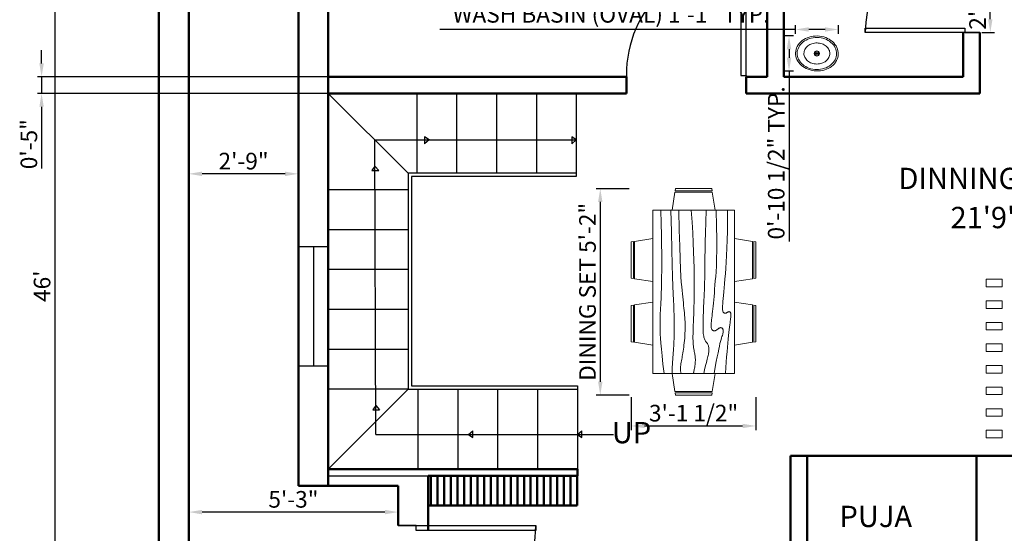
# Model space of a CAD drawing. Units: inches. Extents: x 116541 to 117938, y 135634 to 136328.
# Tile 2 of 9: x 116541 to 116838, y 135936 to 136091. Entities that reach past the tile are written whole.
import ezdxf

# ---------------------------------------------------------------- set-up
doc = ezdxf.new("R2010")
doc.units = ezdxf.units.IN
for name, color, linetype, lineweight in [('A-ANNO-DIMS', 2, 'Continuous', 18), ('A-ANNO-TEXT', 7, 'Continuous', 25), ('A-AREA-IDEN', 3, 'Continuous', 25), ('A-DOOR', 4, 'Continuous', 25), ('A-FLOR-FIXT', 9, 'Continuous', 18), ('A-FLOR-STRS', 2, 'Continuous', 25), ('A-FURN', 8, 'Continuous', 18), ('A-GLAZ', 1, 'Continuous', 25), ('A-WALL', 7, 'Continuous', 50)]:
    doc.layers.add(name, color=color, linetype=linetype, lineweight=lineweight)
doc.styles.get("Standard").update_dxf_attribs({"font": 'arial.ttf'})
doc.dimstyles.new('ISO-25', dxfattribs={"dimtxt": 5, "dimasz": 4, "dimexe": 1.25, "dimexo": 0.625, "dimtad": 1, "dimdec": 3, "dimlunit": 3, "dimtxsty": 'Standard', "dimcen": 2.5, "dimadec": 0, "dimazin": 0, "dimtfac": 1, "dimtdec": 3, "dimtmove": 0, "dimatfit": 3, "dimfxl": 1, "dimarcsym": 0})

# ---------------------------------------------------------------- blocks, each defined once
blk = doc.blocks.new('*U3')
for p, q in [((0, 0), (0, -6)), ((-40, 0), (-40, -6))]:
    blk.add_line(p, q)
blk.add_lwpolyline([(0, 0), (0, 40), (-1.75, 40), (-1.75, 0)], close=True)
blk.add_arc((0, 0), 40, 90, 180)
blk = doc.blocks.new('*U4')
for p, q in [((-40, 0), (-40, 6)), ((0, 0), (0, 6))]:
    blk.add_line(p, q)
blk.add_lwpolyline([(0, 0), (0, -40), (-1.75, -40), (-1.75, 0)], close=True)
blk.add_arc((0, 0), 40, 180, 270)
blk = doc.blocks.new('*U2')
for p, q in [((0, 0), (0, -6)), ((40, 0), (40, -6))]:
    blk.add_line(p, q)
blk.add_lwpolyline([(0, 0), (0, 40), (1.75, 40), (1.75, 0)], close=True)
blk.add_arc((0, 0), 40, 0, 90)
blk = doc.blocks.new('Sink - Oval top')
for p, q in [((-1, 0), (1, 0)), ((0, 1), (0, -1))]:
    blk.add_line(p, q)
for points in [[(-12.23, 0.39, 0.117634), (-11.46, -3.36, 0.104469), (-8.88, -6.8, 0.090016), (-5.08, -9.07, 0.08192), (-0.32, -10.02, 0.08192), (4.49, -9.38, 0.090016), (8.42, -7.36, 0.104469), (11.22, -4.09, 0.117634), (12.23, -0.39, 0.117634), (11.46, 3.36, 0.104469), (8.88, 6.8, 0.090016), (5.08, 9.07, 0.08192), (0.32, 10.02, 0.08192), (-4.49, 9.38, 0.090016), (-8.42, 7.36, 0.104469), (-11.22, 4.09, 0.117634)], [(-11.29, 0.16, 0.118622), (-10.52, -3.25, 0.104678), (-8.07, -6.36, 0.089562), (-4.54, -8.37, 0.081185), (-0.13, -9.15, 0.081185), (4.3, -8.49, 0.089562), (7.89, -6.58, 0.104678), (10.42, -3.55, 0.118622), (11.29, -0.16, 0.118622), (10.52, 3.25, 0.104678), (8.07, 6.36, 0.089562), (4.54, 8.37, 0.081185), (0.13, 9.15, 0.081185), (-4.3, 8.49, 0.089562), (-7.89, 6.58, 0.104678), (-10.42, 3.55, 0.118622)], [(-7.42, 0.08, 0.118283), (-6.91, -2.17, 0.104607), (-5.29, -4.21, 0.089718), (-2.97, -5.53, 0.081436), (-0.07, -6.04, 0.081436), (2.84, -5.59, 0.089718), (5.2, -4.33, 0.104607), (6.86, -2.32, 0.118283), (7.42, -0.08, 0.118283), (6.91, 2.17, 0.104607), (5.29, 4.21, 0.089718), (2.97, 5.53, 0.081436), (0.07, 6.04, 0.081436), (-2.84, 5.59, 0.089718), (-5.2, 4.33, 0.104607), (-6.86, 2.32, 0.118283)]]:
    blk.add_lwpolyline(points, format="xyb", close=True)
for radius in [1.5, 1]:
    blk.add_circle((0, 0), radius)
blk = doc.blocks.new('Dining Set - 36 x 72 in.')
for p, q in [((-22, 27.5), (-22.1562, 26.50042)), ((-5.8416, 26.5), (-22.1534, 26.5)), ((-22, 27.5), (-6, 27.5)), ((-5.8437, 26.49966), (-6, 27.5)), ((6, 27.5), (5.8438, 26.50042)), ((22.1584, 26.5), (5.8466, 26.5)), ((6, 27.5), (22, 27.5)), ((22.1563, 26.49966), (22, 27.5)), ((-22.2343, 26.00059), (-23.4847, 17.99762)), ((-22.2304, 26), (-5.7608, 26)), ((-4.5152, 17.99762), (-5.7655, 25.99926)), ((5.7657, 26.00059), (4.5153, 17.99762)), ((5.7696, 26), (22.2392, 26)), ((23.4848, 17.99762), (22.2345, 25.99926)), ((36, 18), (-36, 18)), ((-36, 18), (-36, -18)), ((36, -18), (36, 18)), ((-44.0006, 8.23428), (-35.9976, 9.48474)), ((44.0006, 8.23428), (35.9976, 9.48474)), ((-45.5, 8), (-44.5004, 8.15617)), ((-45.5, 8), (-45.5, -8)), ((-44.5, -8.15843), (-44.5, 8.15338)), ((-44, 8.23041), (-44, -8.23915)), ((44, 8.23041), (44, -8.23915)), ((44.5, -8.15843), (44.5, 8.15338)), ((45.5, 8), (44.5005, 8.15617)), ((45.5, 8), (45.5, -8)), ((-44.4997, -8.15631), (-45.5, -8)), ((-35.9976, -9.48476), (-43.9993, -8.2345)), ((35.9976, -9.48476), (43.9993, -8.2345)), ((44.4997, -8.15631), (45.5, -8)), ((-36, -18), (36, -18)), ((-22.2343, -26.0006), (-23.4847, -17.99762)), ((-4.5152, -17.99762), (-5.7655, -25.99928)), ((5.7657, -26.0006), (4.5153, -17.99762)), ((23.4848, -17.99762), (22.2345, -25.99928)), ((-22.2304, -26), (-5.7608, -26)), ((5.7696, -26), (22.2392, -26)), ((-22, -27.5), (-22.1562, -26.50044)), ((-5.8416, -26.5), (-22.1534, -26.5)), ((-22, -27.5), (-6, -27.5)), ((-5.8437, -26.49967), (-6, -27.5)), ((6, -27.5), (5.8438, -26.50044)), ((22.1584, -26.5), (5.8466, -26.5)), ((6, -27.5), (22, -27.5)), ((22.1563, -26.49967), (22, -27.5))]:
    blk.add_line(p, q)
for points in [[(-36, 15), (-31.1772, 14.97754), (-26.8079, 14.91406), (-22.8538, 14.81543), (-19.276, 14.6875), (-16.0362, 14.53613), (-13.0957, 14.36718), (-10.4159, 14.18652), (-7.9583, 14), (-5.6904, 13.81315), (-3.6035, 13.63021), (-1.6954, 13.45508), (0.0365, 13.29166), (1.5945, 13.14388), (2.9811, 13.01562), (4.1988, 12.9108), (5.25, 12.83333), (6.1393, 12.78613), (6.8802, 12.76823), (7.4883, 12.77767), (7.9792, 12.8125), (8.3685, 12.87077), (8.6719, 12.95052), (8.9049, 13.0498), (9.0833, 13.16666), (9.2205, 13.29899), (9.3216, 13.44401), (9.3895, 13.59879), (9.4271, 13.76041), (9.4373, 13.92594), (9.4232, 14.09245), (9.3875, 14.257), (9.3333, 14.41666), (9.2638, 14.56917), (9.1836, 14.71484), (9.0975, 14.85465), (9.0104, 14.98958), (8.9272, 15.1206), (8.8529, 15.2487), (8.7922, 15.37483), (8.75, 15.5), (8.7305, 15.62467), (8.7344, 15.74739), (8.7617, 15.86621), (8.8125, 15.97916), (8.8867, 16.08431), (8.9844, 16.17968), (9.1055, 16.26334), (9.25, 16.33333), (9.4189, 16.38802), (9.6172, 16.42708), (9.8506, 16.45052), (10.125, 16.45833), (10.4463, 16.45052), (10.8203, 16.42708), (11.2529, 16.38802), (11.75, 16.33333), (12.3184, 16.26318), (12.9694, 16.17838), (13.7151, 16.07991), (14.5677, 15.96875), (15.5395, 15.84586), (16.6426, 15.71224), (17.8893, 15.56884), (19.2917, 15.41666), (20.859, 15.25667), (22.5879, 15.08984), (24.4721, 14.91715), (26.5052, 14.73958), (28.6809, 14.5581), (30.9929, 14.3737), (33.4347, 14.18733), (36, 14)], [(-36, 10), (-28.9766, 10.14274), (-23.1725, 10.20442), (-18.4241, 10.19775), (-14.5677, 10.13541), (-11.4399, 10.03011), (-8.877, 9.89453), (-6.7154, 9.74137), (-4.7917, 9.58333), (-2.9698, 9.43082), (-1.2246, 9.28515), (0.4415, 9.14534), (2.026, 9.01041), (3.5266, 8.87939), (4.9408, 8.7513), (6.266, 8.62516), (7.5, 8.5), (8.6411, 8.37549), (9.6914, 8.2539), (10.6538, 8.13818), (11.5312, 8.03125), (12.3267, 7.93603), (13.043, 7.85547), (13.6831, 7.79248), (14.25, 7.75), (14.7471, 7.7303), (15.1797, 7.73307), (15.5537, 7.75732), (15.875, 7.80208), (16.1494, 7.86637), (16.3828, 7.94922), (16.5811, 8.04964), (16.75, 8.16666), (16.8944, 8.29915), (17.0143, 8.44531), (17.1089, 8.60319), (17.1771, 8.77083), (17.218, 8.94629), (17.2305, 9.1276), (17.2137, 9.31282), (17.1667, 9.5), (17.0895, 9.6875), (16.987, 9.875), (16.8649, 10.0625), (16.7292, 10.25), (16.5856, 10.4375), (16.4401, 10.625), (16.2985, 10.8125), (16.1667, 11), (16.05, 11.18733), (15.9518, 11.3737), (15.8752, 11.5581), (15.8229, 11.73958), (15.798, 11.91715), (15.8034, 12.08984), (15.842, 12.25667), (15.9167, 12.41666), (16.0295, 12.56836), (16.1784, 12.70833), (16.3605, 12.83268), (16.5729, 12.9375), (16.8127, 13.01888), (17.0768, 13.07291), (17.3625, 13.0957), (17.6667, 13.08333), (17.9894, 13.03312), (18.3418, 12.94726), (18.7382, 12.82918), (19.1927, 12.68229), (19.7195, 12.51001), (20.3327, 12.31575), (21.0465, 12.10294), (21.875, 11.875), (22.8357, 11.63354), (23.959, 11.37304), (25.2786, 11.08618), (26.8282, 10.76562), (28.6414, 10.40405), (30.752, 9.99414), (33.1936, 9.52856), (36, 9)], [(-36, 5.5), (-30.7157, 5.3348), (-26.069, 5.20963), (-21.9946, 5.11767), (-18.4271, 5.05208), (-15.3009, 5.00602), (-12.5508, 4.97265), (-10.1112, 4.94515), (-7.9167, 4.91666), (-5.909, 4.88167), (-4.0586, 4.83984), (-2.3429, 4.79215), (-0.7396, 4.73958), (0.7739, 4.6831), (2.22, 4.6237), (3.6213, 4.56233), (5, 4.5), (6.373, 4.43782), (7.7344, 4.3776), (9.0723, 4.32129), (10.375, 4.27083), (11.6309, 4.22819), (12.8281, 4.19531), (13.9551, 4.17415), (15, 4.16666), (15.954, 4.17448), (16.819, 4.19791), (17.6001, 4.23698), (18.3021, 4.29166), (18.9299, 4.36198), (19.4883, 4.44791), (19.9823, 4.54948), (20.4167, 4.66666), (20.7969, 4.79899), (21.1302, 4.94401), (21.4245, 5.09879), (21.6875, 5.26041), (21.9271, 5.42594), (22.1511, 5.59245), (22.3672, 5.757), (22.5834, 5.91666), (22.8065, 6.06868), (23.0404, 6.21093), (23.2879, 6.34147), (23.5521, 6.45833), (23.8358, 6.55957), (24.142, 6.64323), (24.4735, 6.70735), (24.8334, 6.75), (25.2235, 6.76969), (25.642, 6.76692), (26.0858, 6.74267), (26.5521, 6.69791), (27.0379, 6.63362), (27.5404, 6.55078), (28.0565, 6.45036), (28.5834, 6.33333), (29.1242, 6.19987), (29.7071, 6.04687), (30.3661, 5.87044), (31.1354, 5.66666), (32.0493, 5.43164), (33.142, 5.16146), (34.4475, 4.85221), (36, 4.5)], [(-36, -1), (-30.7915, -0.6591), (-26.0195, -0.38216), (-21.6519, -0.16284), (-17.6563, 0.00521), (-14.0005, 0.12833), (-10.6523, 0.21289), (-7.5796, 0.26522), (-4.75, 0.29166), (-2.134, 0.29793), (0.2878, 0.28711), (2.5317, 0.26163), (4.6146, 0.22396), (6.5529, 0.17651), (8.3633, 0.12174), (10.0623, 0.06209), (11.6667, 0), (13.1899, -0.06201), (14.6341, -0.1211), (15.9982, -0.17432), (17.2813, -0.21875), (18.4823, -0.25147), (19.6003, -0.26953), (20.6343, -0.27002), (21.5834, -0.25), (22.4481, -0.20768), (23.2357, -0.14584), (23.9549, -0.06836), (24.6146, 0.02083), (25.2235, 0.11784), (25.7904, 0.21875), (26.3241, 0.31966), (26.8334, 0.41666), (27.3265, 0.50618), (27.8099, 0.58593), (28.2894, 0.65397), (28.7709, 0.70833), (29.2601, 0.74707), (29.763, 0.76823), (30.2855, 0.76985), (30.8334, 0.75), (31.4088, 0.70784), (31.9994, 0.64713), (32.589, 0.57275), (33.1615, 0.48958), (33.7008, 0.4025), (34.1908, 0.3164), (34.6153, 0.23616), (34.9584, 0.16666), (35.2099, 0.11165), (35.3848, 0.07031), (35.504, 0.04069), (35.5886, 0.02083), (35.6594, 0.00879), (35.7377, 0.0026), (35.8442, 0.00032), (36, 0)], [(-36, -6.5), (-27.1843, -6.31267), (-20.084, -6.1263), (-14.469, -5.9419), (-10.1094, -5.76042), (-6.7752, -5.58285), (-4.2363, -5.41016), (-2.2629, -5.24333), (-0.625, -5.08334), (0.8708, -4.93099), (2.2715, -4.78646), (3.5872, -4.64974), (4.8281, -4.52084), (6.0046, -4.39974), (7.127, -4.28646), (8.2053, -4.18099), (9.25, -4.08334), (10.2705, -3.99382), (11.2734, -3.91407), (12.2647, -3.84603), (13.25, -3.79167), (14.2354, -3.75293), (15.2266, -3.73177), (16.2295, -3.73015), (17.25, -3.75), (18.2912, -3.79248), (19.3451, -3.85547), (20.4009, -3.93604), (21.4479, -4.03125), (22.4754, -4.13819), (23.4727, -4.25391), (24.4289, -4.37549), (25.3334, -4.5), (26.1785, -4.62492), (26.9694, -4.74935), (27.7145, -4.87281), (28.4219, -4.99479), (29.1, -5.11483), (29.7572, -5.23242), (30.4016, -5.34709), (31.0417, -5.45834), (31.6837, -5.56437), (32.3262, -5.65821), (32.9658, -5.73153), (33.599, -5.77604), (34.2224, -5.78345), (34.8327, -5.74545), (35.4264, -5.65373), (36, -5.5)], [(-36, -10), (-26.4022, -9.81299), (-18.4675, -9.62891), (-11.9839, -9.45069), (-6.7396, -9.28125), (-2.5226, -9.12354), (0.8789, -8.98047), (3.6769, -8.85498), (6.0833, -8.75), (8.2767, -8.66765), (10.3021, -8.60677), (12.1712, -8.56543), (13.8958, -8.54167), (15.4876, -8.53353), (16.9583, -8.53907), (18.3197, -8.55632), (19.5834, -8.58334), (20.7616, -8.61841), (21.8685, -8.66081), (22.9188, -8.71004), (23.9271, -8.76563), (24.9081, -8.82707), (25.8763, -8.89388), (26.8465, -8.96558), (27.8334, -9.04167), (28.8474, -9.12118), (29.8828, -9.20117), (30.93, -9.27824), (31.9792, -9.34896), (33.0205, -9.40991), (34.0443, -9.45768), (35.0407, -9.48885), (36, -9.5)], [(-36, -14.5), (-30.0881, -14.33513), (-25.0332, -14.21224), (-20.7312, -14.12647), (-17.0781, -14.07292), (-13.97, -14.04671), (-11.3027, -14.04297), (-8.9724, -14.05681), (-6.875, -14.08334), (-4.9224, -14.11833), (-3.0905, -14.16016), (-1.3709, -14.20785), (0.2448, -14.26042), (1.7647, -14.3169), (3.1973, -14.3763), (4.5507, -14.43767), (5.8333, -14.5), (7.0554, -14.5621), (8.235, -14.62175), (9.3922, -14.67652), (10.5469, -14.72396), (11.7192, -14.76164), (12.929, -14.78711), (14.1965, -14.79794), (15.5417, -14.79167), (16.9933, -14.76424), (18.6152, -14.70508), (20.4804, -14.60197), (22.6615, -14.44271), (25.2312, -14.21509), (28.2624, -13.9069), (31.8277, -13.50594), (36, -13)]]:
    blk.add_lwpolyline(points)
blk = doc.blocks.new('*D26')
at = {"layer": 'A-ANNO-DIMS', "color": 0, "lineweight": -2, "transparency": 16777216}
for p, q in [((116582.55, 136286.5), (116550.65, 136286.5)), ((116551.9, 136282.5), (116551.9, 135738.5)), ((116582.55, 135734.5), (116550.65, 135734.5))]:
    blk.add_line(p, q, dxfattribs=at)
at = {"layer": 'A-ANNO-DIMS', "color": 0, "transparency": 16777216}
for points in [[(116551.23, 136282.5), (116552.56, 136282.5), (116551.9, 136286.5)], [(116551.23, 135738.5), (116552.56, 135738.5), (116551.9, 135734.5)]]:
    blk.add_solid(points, dxfattribs=at)
at = {"layer": 'Defpoints', "color": 0, "transparency": 16777216}
for p in [(116583.18, 136286.5), (116551.9, 135734.5), (116583.18, 135734.5)]:
    blk.add_point(p, dxfattribs=at)
at = {"layer": 'A-ANNO-DIMS', "color": 0, "transparency": 16777216, "insert": (116548.72, 136010.5), "char_height": 5, "attachment_point": 5, "rotation": 90}
blk.add_mtext("46'", dxfattribs=at)
blk = doc.blocks.new('*D29')
at = {"layer": 'A-ANNO-DIMS', "color": 0, "lineweight": -2, "transparency": 16777216}
for p, q in [((116830.8, 136116.82), (116834.55, 136116.82)), ((116833.3, 136090.82), (116833.3, 136112.82)), ((116830.8, 136086.82), (116834.55, 136086.82))]:
    blk.add_line(p, q, dxfattribs=at)
at = {"layer": 'A-ANNO-DIMS', "color": 0, "transparency": 16777216}
for points in [[(116832.63, 136112.82), (116833.97, 136112.82), (116833.3, 136116.82)], [(116832.63, 136090.82), (116833.97, 136090.82), (116833.3, 136086.82)]]:
    blk.add_solid(points, dxfattribs=at)
at = {"layer": 'Defpoints', "color": 0, "transparency": 16777216}
for p in [(116830.18, 136116.82), (116833.3, 136116.82), (116830.18, 136086.82)]:
    blk.add_point(p, dxfattribs=at)
at = {"layer": 'A-ANNO-DIMS', "color": 0, "transparency": 16777216, "insert": (116830.12, 136101.82), "char_height": 5, "attachment_point": 5, "rotation": 90}
blk.add_mtext('2\'-5.996"', dxfattribs=at)
blk = doc.blocks.new('*D30')
at = {"layer": 'A-ANNO-DIMS', "color": 0, "lineweight": -2, "transparency": 16777216}
for p, q in [((116592.18, 135943.91), (116592.18, 135941.32)), ((116655.18, 135943.91), (116655.18, 135941.32)), ((116651.18, 135942.57), (116596.18, 135942.57))]:
    blk.add_line(p, q, dxfattribs=at)
at = {"layer": 'A-ANNO-DIMS', "color": 0, "transparency": 16777216}
for points in [[(116596.18, 135943.23), (116596.18, 135941.9), (116592.18, 135942.57)], [(116651.18, 135943.23), (116651.18, 135941.9), (116655.18, 135942.57)]]:
    blk.add_solid(points, dxfattribs=at)
at = {"layer": 'Defpoints', "color": 0, "transparency": 16777216}
for p in [(116592.18, 135944.54), (116655.18, 135944.54), (116592.18, 135942.57)]:
    blk.add_point(p, dxfattribs=at)
at = {"layer": 'A-ANNO-DIMS', "color": 0, "transparency": 16777216, "insert": (116623.68, 135945.75), "char_height": 5, "attachment_point": 5}
blk.add_mtext('5\'-3"', dxfattribs=at)
blk = doc.blocks.new('*D31')
at = {"layer": 'A-ANNO-DIMS', "color": 0, "lineweight": -2, "transparency": 16777216}
for p, q in [((116592.18, 136044.94), (116592.18, 136045.56)), ((116625.18, 136044.94), (116625.18, 136045.56)), ((116621.18, 136044.31), (116596.18, 136044.31))]:
    blk.add_line(p, q, dxfattribs=at)
at = {"layer": 'A-ANNO-DIMS', "color": 0, "transparency": 16777216}
for points in [[(116596.18, 136044.98), (116596.18, 136043.64), (116592.18, 136044.31)], [(116621.18, 136044.98), (116621.18, 136043.64), (116625.18, 136044.31)]]:
    blk.add_solid(points, dxfattribs=at)
at = {"layer": 'Defpoints', "color": 0, "transparency": 16777216}
for p in [(116592.18, 136044.31), (116592.18, 136044.31), (116625.18, 136044.31)]:
    blk.add_point(p, dxfattribs=at)
at = {"layer": 'A-ANNO-DIMS', "color": 0, "transparency": 16777216, "insert": (116608.68, 136047.49), "char_height": 5, "attachment_point": 5}
blk.add_mtext('2\'-9"', dxfattribs=at)
blk = doc.blocks.new('*D62')
at = {"layer": 'A-ANNO-DIMS', "color": 0, "lineweight": -2, "transparency": 16777216}
for p, q in [((116774.69, 136086.42), (116774.69, 136088.98)), ((116787.59, 136086.42), (116787.59, 136088.98)), ((116774.69, 136087.73), (116667.73, 136087.73)), ((116783.59, 136087.73), (116778.69, 136087.73))]:
    blk.add_line(p, q, dxfattribs=at)
at = {"layer": 'A-ANNO-DIMS', "color": 0, "transparency": 16777216}
for points in [[(116778.69, 136088.4), (116778.69, 136087.07), (116774.69, 136087.73)], [(116783.59, 136088.4), (116783.59, 136087.07), (116787.59, 136087.73)]]:
    blk.add_solid(points, dxfattribs=at)
at = {"layer": 'Defpoints', "color": 0, "transparency": 16777216}
for p in [(116774.69, 136087.73), (116774.69, 136085.8), (116787.59, 136085.8)]:
    blk.add_point(p, dxfattribs=at)
at = {"layer": 'A-ANNO-DIMS', "color": 0, "transparency": 16777216, "insert": (116719.21, 136091.64), "char_height": 5, "attachment_point": 5}
blk.add_mtext('WASH BASIN (OVAL) 1\'-1" TYP.', dxfattribs=at)
blk = doc.blocks.new('*D63')
at = {"layer": 'A-ANNO-DIMS', "color": 0, "lineweight": -2, "transparency": 16777216}
for p, q in [((116774.07, 136085.8), (116771.51, 136085.8)), ((116772.76, 136081.8), (116772.76, 136079.22)), ((116774.07, 136075.22), (116771.51, 136075.22)), ((116772.76, 136075.22), (116772.76, 136023.96))]:
    blk.add_line(p, q, dxfattribs=at)
at = {"layer": 'A-ANNO-DIMS', "color": 0, "transparency": 16777216}
for points in [[(116772.09, 136081.8), (116773.43, 136081.8), (116772.76, 136085.8)], [(116772.09, 136079.22), (116773.43, 136079.22), (116772.76, 136075.22)]]:
    blk.add_solid(points, dxfattribs=at)
at = {"layer": 'Defpoints', "color": 0, "transparency": 16777216}
for p in [(116774.69, 136085.8), (116772.76, 136075.22), (116774.69, 136075.22)]:
    blk.add_point(p, dxfattribs=at)
at = {"layer": 'A-ANNO-DIMS', "color": 0, "transparency": 16777216, "insert": (116769.55, 136047.59), "char_height": 5, "attachment_point": 5, "rotation": 90}
blk.add_mtext('0\'-10 1/2" TYP.', dxfattribs=at)
blk = doc.blocks.new('*D78')
at = {"layer": 'A-ANNO-DIMS', "color": 0, "lineweight": -2, "transparency": 16777216}
for p, q in [((116724.67, 136039.85), (116714.74, 136039.85)), ((116715.99, 136035.85), (116715.99, 135981.78)), ((116724.67, 135977.78), (116714.74, 135977.78))]:
    blk.add_line(p, q, dxfattribs=at)
at = {"layer": 'A-ANNO-DIMS', "color": 0, "transparency": 16777216}
for points in [[(116715.32, 136035.85), (116716.65, 136035.85), (116715.99, 136039.85)], [(116715.32, 135981.78), (116716.65, 135981.78), (116715.99, 135977.78)]]:
    blk.add_solid(points, dxfattribs=at)
at = {"layer": 'Defpoints', "color": 0, "transparency": 16777216}
for p in [(116725.3, 136039.85), (116715.99, 135977.78), (116725.3, 135977.78)]:
    blk.add_point(p, dxfattribs=at)
at = {"layer": 'A-ANNO-DIMS', "color": 0, "transparency": 16777216, "insert": (116712.78, 136008.82), "char_height": 5, "attachment_point": 5, "rotation": 90}
blk.add_mtext('DINING SET 5\'-2"', dxfattribs=at)
blk = doc.blocks.new('*D79')
at = {"layer": 'A-ANNO-DIMS', "color": 0, "lineweight": -2, "transparency": 16777216}
for p, q in [((116725.3, 135977.16), (116725.3, 135967.22)), ((116762.81, 135977.16), (116762.81, 135967.22)), ((116729.3, 135968.47), (116758.81, 135968.47))]:
    blk.add_line(p, q, dxfattribs=at)
at = {"layer": 'A-ANNO-DIMS', "color": 0, "transparency": 16777216}
for points in [[(116729.3, 135969.14), (116729.3, 135967.81), (116725.3, 135968.47)], [(116758.81, 135969.14), (116758.81, 135967.81), (116762.81, 135968.47)]]:
    blk.add_solid(points, dxfattribs=at)
at = {"layer": 'Defpoints', "color": 0, "transparency": 16777216}
for p in [(116725.3, 135977.78), (116762.81, 135977.78), (116762.81, 135968.47)]:
    blk.add_point(p, dxfattribs=at)
at = {"layer": 'A-ANNO-DIMS', "color": 0, "transparency": 16777216, "insert": (116744.05, 135971.68), "char_height": 5, "attachment_point": 5}
blk.add_mtext('3\'-1 1/2"', dxfattribs=at)
blk = doc.blocks.new('*D106')
at = {"layer": 'A-ANNO-DIMS', "color": 0, "lineweight": -2, "transparency": 16777216}
for p, q in [((116547.93, 136077.5), (116547.93, 136081.5)), ((116723.2, 136073.5), (116546.68, 136073.5)), ((116547.93, 136073.5), (116547.93, 136068.5)), ((116723.2, 136068.5), (116546.68, 136068.5)), ((116547.93, 136064.5), (116547.93, 136045.96))]:
    blk.add_line(p, q, dxfattribs=at)
at = {"layer": 'A-ANNO-DIMS', "color": 0, "transparency": 16777216}
for points in [[(116547.26, 136077.5), (116548.59, 136077.5), (116547.93, 136073.5)], [(116547.26, 136064.5), (116548.59, 136064.5), (116547.93, 136068.5)]]:
    blk.add_solid(points, dxfattribs=at)
at = {"layer": 'Defpoints', "color": 0, "transparency": 16777216}
for p in [(116723.83, 136073.5), (116547.93, 136068.5), (116723.83, 136068.5)]:
    blk.add_point(p, dxfattribs=at)
at = {"layer": 'A-ANNO-DIMS', "color": 0, "transparency": 16777216, "insert": (116544.75, 136053.23), "char_height": 5, "attachment_point": 5, "rotation": 90}
blk.add_mtext('0\'-5"', dxfattribs=at)

msp = doc.modelspace()

# ---------------------------------------------------------------- linework, layer by layer
at = {"layer": 'A-DOOR'}
for points in [[(116830.1763, 136086.8229), (116825.1763, 136086.8229)], [(116655.1763, 135938.5688), (116664.1763, 135938.5688), (116664.1763, 135936.9938)]]:
    msp.add_lwpolyline(points, dxfattribs=at)
at = {"layer": 'A-FLOR-STRS'}
for p, q in [((116708.7773, 136068.5034), (116634.1763, 136068.5034)), ((116634.1763, 136068.5034), (116634.1763, 135955.5034)), ((116658.1763, 136044.5034), (116634.1763, 136068.5034)), ((116660.7773, 136068.5034), (116660.7773, 136044.5034)), ((116672.7773, 136068.5034), (116672.7773, 136044.5034)), ((116684.7773, 136068.5034), (116684.7773, 136044.5034)), ((116696.7773, 136068.5034), (116696.7773, 136044.5034)), ((116708.7773, 136068.5034), (116708.7773, 136044.5034)), ((116648.4737, 135965.9009), (116648.1767, 136054.5031)), ((116648.1767, 136054.5031), (116708.7773, 136054.5031)), ((116664.5169, 136054.5031), (116663.156, 136055.4271)), ((116663.156, 136055.4271), (116663.156, 136053.3546)), ((116664.5169, 136054.5031), (116663.156, 136053.3546)), ((116708.7773, 136054.5031), (116707.4164, 136055.4271)), ((116707.4164, 136055.4271), (116707.4164, 136053.3546)), ((116708.7773, 136054.5031), (116707.4164, 136053.3546)), ((116648.203, 136046.6422), (116647.2789, 136045.2813)), ((116647.2789, 136045.2813), (116649.3515, 136045.2813)), ((116648.203, 136046.6422), (116649.3515, 136045.2813)), ((116708.7773, 136044.5034), (116658.1763, 136044.5034)), ((116658.1763, 136044.5034), (116658.1763, 135979.5034)), ((116708.7773, 136044.5034), (116708.7773, 136043.5034)), ((116659.1763, 136043.5034), (116659.1763, 135980.5034)), ((116708.7773, 136043.5034), (116659.1763, 136043.5034)), ((116658.1763, 136039.5034), (116634.1763, 136039.5034)), ((116658.1763, 136027.5034), (116634.1763, 136027.5034)), ((116658.1763, 136015.5034), (116634.1763, 136015.5034)), ((116658.1763, 136003.5034), (116634.1763, 136003.5034)), ((116658.1763, 135991.5034), (116634.1763, 135991.5034)), ((116658.1763, 135979.5034), (116634.1763, 135955.5034)), ((116658.1763, 135979.5034), (116634.1763, 135979.5034)), ((116658.1763, 135979.5034), (116709.0888, 135979.5034)), ((116659.1763, 135980.5034), (116709.0888, 135980.5034)), ((116661.0888, 135979.5034), (116661.0888, 135955.5034)), ((116673.0888, 135979.5034), (116673.0888, 135955.5034)), ((116685.0888, 135979.5034), (116685.0888, 135955.5034)), ((116697.0888, 135979.5034), (116697.0888, 135955.5034)), ((116709.0888, 135980.5034), (116709.0888, 135979.5034)), ((116709.0888, 135979.5034), (116709.0888, 135955.5034)), ((116648.4443, 135974.6742), (116647.5202, 135973.3133)), ((116648.4443, 135974.6742), (116649.5928, 135973.3133)), ((116647.5202, 135973.3133), (116649.5928, 135973.3133)), ((116648.4737, 135965.9009), (116719.9549, 135965.9009)), ((116676.2959, 135965.9009), (116677.6568, 135967.0493)), ((116676.2959, 135965.9009), (116677.6568, 135964.9768)), ((116677.6568, 135964.9768), (116677.6568, 135967.0493)), ((116709.0888, 135965.9009), (116710.4497, 135967.0493)), ((116709.0888, 135965.9009), (116710.4497, 135964.9768)), ((116710.4497, 135964.9768), (116710.4497, 135967.0493)), ((116634.1763, 135955.5034), (116709.0888, 135955.5034)), ((116634.1763, 135953.5034), (116709.0888, 135953.5034))]:
    msp.add_line(p, q, dxfattribs=at)
at = {"layer": 'A-FURN'}
for points in [[(116832.0161, 136012.5959), (116836.8536, 136012.5959), (116836.8536, 136010.341), (116832.0161, 136010.341)], [(116832.0161, 136006.107), (116836.8536, 136006.107), (116836.8536, 136003.8521), (116832.0161, 136003.8521)], [(116832.0161, 135999.6181), (116836.8536, 135999.6181), (116836.8536, 135997.3632), (116832.0161, 135997.3632)], [(116832.0161, 135993.1291), (116836.8536, 135993.1291), (116836.8536, 135990.8743), (116832.0161, 135990.8743)], [(116832.0161, 135986.6402), (116836.8536, 135986.6402), (116836.8536, 135984.3853), (116832.0161, 135984.3853)], [(116832.0161, 135980.1513), (116836.8536, 135980.1513), (116836.8536, 135977.8964), (116832.0161, 135977.8964)], [(116832.0161, 135973.6624), (116836.8536, 135973.6624), (116836.8536, 135971.4075), (116832.0161, 135971.4075)], [(116832.0161, 135967.1735), (116836.8536, 135967.1735), (116836.8536, 135964.9186), (116832.0161, 135964.9186)]]:
    msp.add_lwpolyline(points, close=True, dxfattribs=at)
at = {"layer": 'A-GLAZ'}
msp.add_line((116629.6763, 136022.4398), (116629.6763, 135986.4398), dxfattribs=at)
msp.add_lwpolyline([(116625.1763, 136022.4398), (116634.1763, 136022.4398), (116634.1763, 135986.4398), (116625.1763, 135986.4398)], close=True, dxfattribs=at)
at = {"layer": 'A-WALL'}
for p, q in [((116583.1763, 136286.5034), (116583.1763, 135734.5034)), ((116592.1763, 136277.5034), (116592.1763, 135743.5034)), ((116625.1763, 136244.5034), (116625.1763, 135950.5034)), ((116634.1763, 136235.5034), (116634.1763, 135950.5034)), ((116766.1763, 136196.5704), (116766.1763, 136073.5034)), ((116771.1763, 136129.0034), (116771.1763, 136073.5034)), ((116825.1763, 136086.8229), (116825.1763, 136073.5034)), ((116830.1763, 136086.8229), (116830.1763, 136068.5034)), ((116634.1763, 136073.5034), (116723.8277, 136073.5034)), ((116759.8277, 136073.5034), (116766.1763, 136073.5034)), ((116771.1763, 136073.5034), (116825.1763, 136073.5034)), ((116634.1763, 136068.5034), (116723.8277, 136068.5034)), ((116759.8277, 136068.5034), (116830.1763, 136068.5034)), ((116773.1763, 135959.5034), (116923.6763, 135959.5034)), ((116773.1763, 135955.5034), (116773.1763, 135959.5034)), ((116778.1763, 135955.5034), (116778.1763, 135959.5034)), ((116829.1763, 135955.5034), (116829.1763, 135959.5034)), ((116634.1763, 135955.5034), (116709.0888, 135955.5034)), ((116664.1763, 135953.5034), (116709.0418, 135953.5034)), ((116664.1763, 135944.5316), (116664.1763, 135953.5034)), ((116665.0418, 135953.5034), (116665.0418, 135944.5316)), ((116667.0418, 135953.5034), (116667.0418, 135944.5316)), ((116669.0418, 135953.5034), (116669.0418, 135944.5316)), ((116671.0418, 135953.5034), (116671.0418, 135944.5316)), ((116673.0418, 135953.5034), (116673.0418, 135944.5316)), ((116675.0418, 135953.5034), (116675.0418, 135944.5316)), ((116677.0418, 135953.5034), (116677.0418, 135944.5316)), ((116677.0418, 135953.5034), (116677.0418, 135944.5316)), ((116679.0418, 135953.5034), (116679.0418, 135944.5316)), ((116681.0418, 135953.5034), (116681.0418, 135944.5316)), ((116683.0418, 135953.5034), (116683.0418, 135944.5316)), ((116685.0418, 135953.5034), (116685.0418, 135944.5316)), ((116687.0418, 135953.5034), (116687.0418, 135944.5316)), ((116689.0418, 135953.5034), (116689.0418, 135944.5316)), ((116691.0418, 135953.5034), (116691.0418, 135944.5316)), ((116693.0418, 135953.5034), (116693.0418, 135944.5316)), ((116695.0418, 135953.5034), (116695.0418, 135944.5316)), ((116697.0418, 135953.5034), (116697.0418, 135944.5316)), ((116699.0418, 135953.5034), (116699.0418, 135944.5316)), ((116701.0418, 135953.5034), (116701.0418, 135944.5316)), ((116703.0418, 135953.5034), (116703.0418, 135944.5316)), ((116705.0418, 135953.5034), (116705.0418, 135944.5316)), ((116707.0418, 135953.5034), (116707.0418, 135944.5316)), ((116709.0418, 135953.5034), (116709.0418, 135944.5316)), ((116709.0888, 135953.5034), (116709.0888, 135955.5034)), ((116773.1763, 135955.5034), (116773.1763, 135902.0034)), ((116778.1763, 135955.5034), (116778.1763, 135907.0034)), ((116829.1763, 135955.5034), (116829.1763, 135806.5034)), ((116625.1763, 135950.5034), (116655.1763, 135950.5034)), ((116655.1763, 135938.5688), (116655.1763, 135950.5034)), ((116664.1763, 135936.9938), (116664.1763, 135950.5034)), ((116709.0418, 135944.5316), (116664.1763, 135944.5316))]:
    msp.add_line(p, q, dxfattribs=at)
for points in [[(116723.8277, 136068.5034), (116723.8277, 136073.5034)], [(116759.8277, 136073.5034), (116759.8277, 136068.5034)]]:
    msp.add_lwpolyline(points, dxfattribs=at)
msp.add_lwpolyline([(116664.1763, 135953.5034), (116709.0888, 135953.5034), (116709.0888, 135953.5034), (116664.1763, 135953.5034)], close=True, dxfattribs=at)

# ---------------------------------------------------------------- block references
at = {"layer": 'A-DOOR', "rotation": 90}
for name, p, xscale, yscale, zscale in [('*U2', (116825.6769, 136086.8229), 0.749895633020561, 0.749895633020561, 0.749895633020561), ('*U4', (116660.5763, 135938.5688), 0.9, 0.9, 0.9)]:
    msp.add_blockref(name, p, dxfattribs=dict(at, xscale=xscale, yscale=yscale, zscale=zscale))
at = {"layer": 'A-DOOR', "xscale": 0.9, "yscale": 0.9, "zscale": 0.9}
msp.add_blockref('*U3', (116759.8277, 136073.9034), dxfattribs=at)
at = {"layer": 'A-FLOR-FIXT', "xscale": 0.5252454991663538, "yscale": 0.5252454991663538, "zscale": 0.5252454991663538, "rotation": 180}
msp.add_blockref('Sink - Oval top', (116781.1404, 136080.5117), dxfattribs=at)
at = {"layer": 'A-FURN', "xscale": 0.6820736143090995, "yscale": 0.6820736143090995, "zscale": 0.6820736143090995, "rotation": 269.999999999994}
msp.add_blockref('Dining Set - 36 x 72 in.', (116744.0533, 136008.8171), dxfattribs=at)

# ---------------------------------------------------------------- texts
at = {"layer": 'A-ANNO-TEXT'}
msp.add_text('UP', height=6.40837, dxfattribs=at).set_placement((116719.4625, 135963.2732))
at = {"layer": 'A-AREA-IDEN'}
for s, height, p in [('DINNING / DRAWING', 6.408368, (116805.675, 136039.7235)), ('        21\'9"X12\'', 6.408368, (116805.675, 136027.9633)), ('PUJA ', 6.40837, (116787.9392, 135938.0678))]:
    msp.add_text(s, height=height, dxfattribs=at).set_placement(p)

# ---------------------------------------------------------------- dimensions: what is measured, and where the dimension line sits
at = {"layer": 'A-ANNO-DIMS'}
for base, p1, p2, override, picture, middle in [((116551.8967, 135734.5034), (116583.1763, 136286.5034), (116583.1763, 135734.5034), {"dimclrd": 0, "dimclre": 0, "dimclrt": 0}, '*D26', (116548.7188, 136010.5034)), ((116833.2999, 136116.8187), (116830.1763, 136086.8229), (116830.1763, 136116.8187), {"dimclrd": 0, "dimclre": 0, "dimclrt": 0}, '*D29', (116830.1221, 136101.8208)), ((116547.9263, 136068.5034), (116723.8277, 136073.5034), (116723.8277, 136068.5034), {"dimdec": 1, "dimlfac": 1, "dimrnd": 0, "dimzin": 1, "dimdsep": 46, "dimlunit": 4, "dimfrac": 2}, '*D106', (116544.7484, 136053.2328))]:
    dim = msp.add_linear_dim(base=base, p1=p1, p2=p2, angle=90, dimstyle='ISO-25', override=override, dxfattribs=at)
    dim.commit()
    dim.dimension.update_dxf_attribs({"geometry": picture, "text_midpoint": middle})
for base, p1, p2, angle, text, picture, middle in [((116774.6928, 136087.7343), (116787.588, 136085.8), (116774.6928, 136085.8), 180, 'WASH BASIN (OVAL) <> TYP.', '*D62', (116719.2134, 136091.6386)), ((116772.7585, 136075.2233), (116774.6928, 136085.8), (116774.6928, 136075.2233), 270, '<> TYP.', '*D63', (116769.5482, 136047.5919)), ((116715.986, 135977.7827), (116725.2963, 136039.8514), (116725.2963, 135977.7827), 270, 'DINING SET <>', '*D78', (116712.7757, 136008.8171))]:
    dim = msp.add_linear_dim(base=base, p1=p1, p2=p2, angle=angle, text=text, dimstyle='ISO-25', override={"dimdec": 1, "dimrnd": 0, "dimzin": 1, "dimlunit": 4, "dimfrac": 2}, dxfattribs=at)
    dim.commit()
    dim.dimension.update_dxf_attribs({"geometry": picture, "text_midpoint": middle})
for base, p1, p2, override, picture, middle in [((116592.1763, 136044.3116), (116625.1763, 136044.3116), (116592.1763, 136044.3116), {"dimclrd": 0, "dimclre": 0, "dimclrt": 0}, '*D31', (116608.6763, 136047.4895)), ((116762.8103, 135968.4724), (116725.2963, 135977.7827), (116762.8103, 135977.7827), {"dimdec": 1, "dimrnd": 0, "dimzin": 1, "dimlunit": 4, "dimfrac": 2}, '*D79', (116744.0533, 135971.6844)), ((116592.1763, 135942.5668), (116655.1763, 135944.5361), (116592.1763, 135944.5361), {"dimclrd": 0, "dimclre": 0, "dimclrt": 0}, '*D30', (116623.6763, 135945.7463))]:
    dim = msp.add_linear_dim(base=base, p1=p1, p2=p2, dimstyle='ISO-25', override=override, dxfattribs=at)
    dim.commit()
    dim.dimension.update_dxf_attribs({"geometry": picture, "text_midpoint": middle})

doc.saveas('drawing.dxf')
